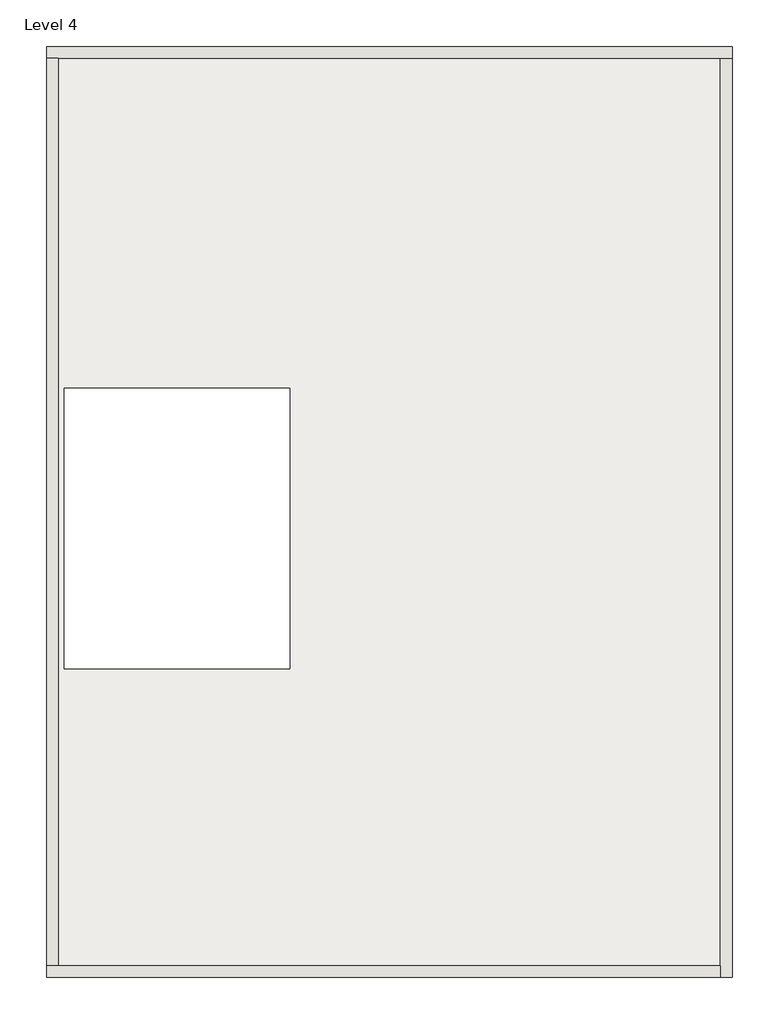
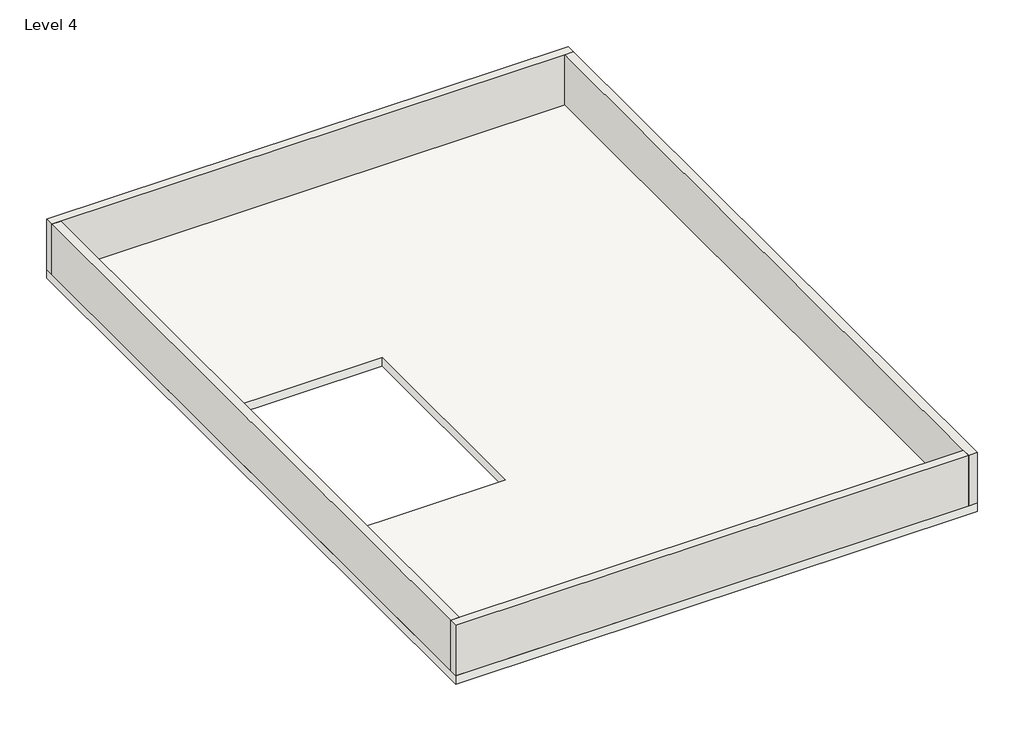
# One storey: 4 walls, 1 roof.
"""IFC4 building model written with IfcOpenShell, lengths in millimetres."""

from ifc_helpers import new_model, si_unit, frame, origin, place, context, project, spatial, polyline, outline, extrude, faceted_brep, element, save

model = new_model("IFC4")

# Units and contexts
model_context = context("Model", 3, world=origin())
ifc_project = project(units=[si_unit("LENGTHUNIT", "METRE", prefix="MILLI")], contexts=[model_context])

# Site, building, storey
site = spatial("IfcSite", under=ifc_project)
building = spatial("IfcBuilding", under=site)
storey = spatial("IfcBuildingStorey", under=building, Name="Level 4", Elevation=9601.2)

# Roof
placement = place(None, origin())
element("IfcRoof", 1, ObjectType="Generic - 12\"", at=placement, inside=storey, context=model_context, shape_type="SweptSolid", body=[
    extrude(outline(polyline([(-22944.8789184, -5144.3399287), (-22944.8789184, 6996.8600713), (-14004.0789184, 6996.8600713), (-14004.0789184, -5144.3399287), (-22944.8789184, -5144.3399287)]), holes=[polyline([(-22716.2789184, 2539.1600713), (-22716.2789184, -1118.4399287), (-19769.8789184, -1118.4399287), (-19769.8789184, 2539.1600713), (-22716.2789184, 2539.1600713)])]), frame((0.0, 0.0, 9296.4), z_axis=(0.0, 0.0, 1.0), x_axis=(1.0, 0.0, 0.0)), (0.0, 0.0, 1.0), 152.4),
])

# Walls
element("IfcWall", 2, ObjectType="parapet wall 3'", at=placement, inside=storey, context=model_context, shape_type="Brep", body=[
    faceted_brep([(-22944.8789184, 6844.4600713, 9448.8), (-22792.4789184, 6844.4600713, 9448.8), (-14156.4789184, 6844.4600713, 9448.8), (-14004.0789184, 6844.4600713, 9448.8), (-14004.0789184, 6844.4600713, 10363.2), (-14156.4789184, 6844.4600713, 10363.2), (-22792.4789184, 6844.4600713, 10363.2), (-22944.8789184, 6844.4600713, 10363.2), (-22944.8789184, 6996.8600713, 9448.8), (-22944.8789184, 6996.8600713, 10363.2), (-14004.0789184, 6996.8600713, 10363.2), (-14004.0789184, 6996.8600713, 9448.8)], [[[0, 1, 2, 3, 4, 5, 6, 7]], [[8, 9, 10, 11]], [[3, 2, 1, 0, 8, 11]], [[7, 6, 5, 4, 10, 9]], [[4, 3, 11, 10]], [[0, 7, 9, 8]]]),
])
element("IfcWall", 3, ObjectType="parapet wall 3'", at=placement, inside=storey, context=model_context, shape_type="Brep", body=[
    faceted_brep([(-14156.4789184, 6844.4600713, 9448.8), (-14156.4789184, -4991.9399287, 9448.8), (-14156.4789184, -5144.3399287, 9448.8), (-14156.4789184, -5144.3399287, 10363.2), (-14156.4789184, -4991.9399287, 10363.2), (-14156.4789184, 6844.4600713, 10363.2), (-14004.0789184, 6844.4600713, 9448.8), (-14004.0789184, 6844.4600713, 10363.2), (-14004.0789184, -5144.3399287, 10363.2), (-14004.0789184, -5144.3399287, 9448.8)], [[[0, 1, 2, 3, 4, 5]], [[6, 7, 8, 9]], [[2, 1, 0, 6, 9]], [[5, 4, 3, 8, 7]], [[0, 5, 7, 6]], [[3, 2, 9, 8]]]),
])
element("IfcWall", 4, ObjectType="parapet wall 3'", at=placement, inside=storey, context=model_context, shape_type="Brep", body=[
    faceted_brep([(-14156.4789184, -4991.9399287, 9448.8), (-22792.4789184, -4991.9399287, 9448.8), (-22944.8789184, -4991.9399287, 9448.8), (-22944.8789184, -4991.9399287, 10363.2), (-22792.4789184, -4991.9399287, 10363.2), (-14156.4789184, -4991.9399287, 10363.2), (-14156.4789184, -5144.3399287, 9448.8), (-14156.4789184, -5144.3399287, 10363.2), (-22944.8789184, -5144.3399287, 10363.2), (-22944.8789184, -5144.3399287, 9448.8)], [[[0, 1, 2, 3, 4, 5]], [[6, 7, 8, 9]], [[2, 1, 0, 6, 9]], [[5, 4, 3, 8, 7]], [[0, 5, 7, 6]], [[3, 2, 9, 8]]]),
])
element("IfcWall", 5, ObjectType="parapet wall 3'", at=placement, inside=storey, context=model_context, shape_type="SweptSolid", body=[
    extrude(outline(polyline([(-22944.8789184, -4991.9399287), (-22944.8789184, 6844.4600713), (-22792.4789184, 6844.4600713), (-22792.4789184, -4991.9399287), (-22944.8789184, -4991.9399287)])), frame((0.0, 0.0, 9448.8), z_axis=(0.0, 0.0, 1.0), x_axis=(1.0, 0.0, 0.0)), (0.0, 0.0, 1.0), 914.4),
])

save(model, "model.ifc")

# Revit data of these elements
# Type "Generic - 12\""
#   Assembly Code = "B1020"
#   Layers, outside or top first: 0' - 6" no material (function 1)
# Type "parapet wall 3'"
#   Assembly Code = "B2010"
#   Layers, outside or top first: 0' - 6" no material (function 1)
# Element 1 (IfcRoof, "Generic - 12\"")
#   built-in parameter 1001705 = 31 (stored number, unit not read)
#   built-in parameter 1001701 = -1 (stored number, unit not read)
#   built-in parameter 1001710 = 33615
#   Phase Created = New Construction
#   Materials on its faces: "light shade", "Default Roof", "Wood - Stained"
# Elements 2, 3, 4 (IfcWall, "parapet wall 3'")
#   built-in parameter 1001111 = -0' - 6"
#   Top Offset = 0' - 0"
#   Base Offset = -0' - 6"
#   Unconnected Height = 3' - 0"
#   wall height = 3' - 0"
#   Phase Created = New Construction
#   Base Constraint = Level 4
#   Materials on its faces: "1 wall", "Default Wall", "Clad - White"
# Element 5 (IfcWall, "parapet wall 3'")
#   built-in parameter 1001111 = -0' - 6"
#   Top Offset = 0' - 0"
#   Base Offset = -0' - 6"
#   Unconnected Height = 3' - 0"
#   wall height = 3' - 0"
#   Phase Created = New Construction
#   Base Constraint = Level 4
#   Materials on its faces: "Default Wall", "1 wall", "Clad - White"
# Materials
#   "light shade": class "Generic", colour RGB 120 120 120, transparency 0, Cost = 0
#   "Default Roof": colour RGB 88 101 114, transparency 0, Cost = 0
#   "Wood - Stained": class "Wood", colour RGB 224 178 126, transparency 0, Cost = 0
#   "1 wall": class "Glass", colour RGB 0 0 255, transparency 0.75, Cost = 0
#   "Default Wall": colour RGB 128 128 128, transparency 0, Cost = 0
#   "Clad - White": class "Wood", colour RGB 242 242 238, transparency 0, Cost = 0
